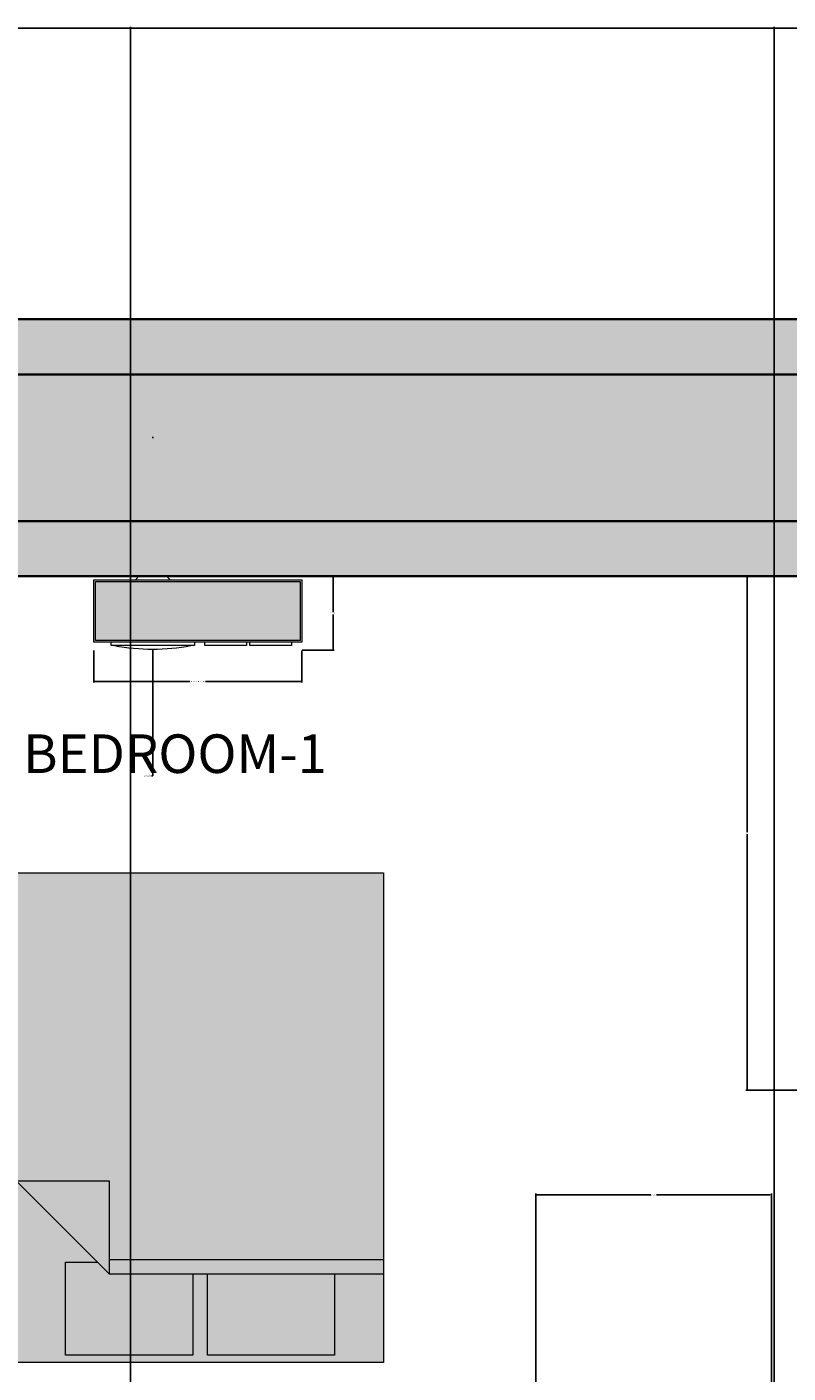
# Model space of a CAD drawing. Units: inches. Extents: x 2549 to 3108, y 1683 to 2362.
# Tile 20 of 30: x 2664 to 2788, y 2142 to 2362. Entities that reach past the tile are written whole.
import ezdxf

# ---------------------------------------------------------------- set-up
doc = ezdxf.new("R2010")
doc.units = ezdxf.units.IN
for name, color, linetype, lineweight in [('A-ANNO-DIMS', 2, 'Continuous', 18), ('A-AREA-IDEN', 7, 'Continuous', 18), ('A-FURN', 8, 'Continuous', 18), ('A-FURN-PATT', 9, 'Continuous', 13), ('A-WALL', 7, 'Continuous', 35), ('A-WALL-PATT', 89, 'Continuous', 13), ('C-PROP', 7, 'Continuous', 35)]:
    doc.layers.add(name, color=color, linetype=linetype, lineweight=lineweight)
for name, color, linetype, lineweight, true_color in [('C-PKNG-VEHI-PATT', 251, 'Continuous', 13, 0x636466), ('C-PROP-PATT', 252, 'Continuous', 13, 0x939598), ('C-PVMT-PATT', 9, 'Continuous', 13, 0xc7c8ca)]:
    doc.layers.add(name, color=color, linetype=linetype, lineweight=lineweight, true_color=true_color)
doc.styles.get("Standard").update_dxf_attribs({"font": 'arial.ttf'})
doc.dimstyles.get("Standard").update_dxf_attribs({"dimtxt": 0.18, "dimasz": 0.18, "dimexe": 0.18, "dimexo": 0.0625, "dimgap": 0.09, "dimtad": 0, "dimtih": 1, "dimtoh": 1, "dimdec": 4, "dimzin": 0, "dimdsep": 46, "dimtxsty": 'Standard', "dimcen": 0.09, "dimadec": 0, "dimazin": 0, "dimtfac": 1, "dimtdec": 4, "dimtofl": 0, "dimtmove": 0, "dimatfit": 3, "dimfxl": 1, "dimtolj": 1, "dimtzin": 0, "dimarcsym": 0})

# ---------------------------------------------------------------- blocks, each defined once
blk = doc.blocks.new('Bed - Queen')
for p, q in [((0, -80.00003), (0, 0)), ((0, 0), (59.99999, 0)), ((59.99999, 0), (59.99999, -80.00003)), ((7.99999, -1.2), (28.79998, -1.2)), ((7.99999, -14.4), (7.99999, -1.2)), ((28.79998, -1.2), (28.79998, -14.4)), ((31.19999, -1.2), (51.99999, -1.2)), ((31.19999, -14.4), (31.19999, -1.2)), ((51.99999, -1.2), (51.99999, -16.4)), ((0, -14.4), (44.8, -14.4)), ((59.99999, -29.6), (44.8, -14.4)), ((44.8, -14.4), (44.8, -29.6)), ((44.8, -16.8), (0, -16.8)), ((51.99999, -16.4), (46.79936, -16.4)), ((44.8, -29.6), (59.99999, -29.6)), ((59.99999, -80.00003), (0, -80.00003))]:
    blk.add_line(p, q)
blk = doc.blocks.new('Entertainment Center')
for p, q in [((-4, 0), (-5, -1)), ((4, 0), (-4, 0)), ((5, -1), (4, 0)), ((-17, -19), (-17, -1)), ((-17, -1), (43, -1)), ((-16.5, -18.5), (-16.5, -1.5)), ((-16.5, -1.5), (42.5, -1.5)), ((42.5, -1.5), (42.5, -18.5)), ((43, -1), (43, -19)), ((43, -19), (-17, -19)), ((42.5, -18.5), (-16.5, -18.5)), ((-12, -20), (-12, -19)), ((12, -19), (12, -20)), ((15, -20), (15, -19)), ((27, -19), (27, -20)), ((28, -20), (28, -19)), ((40, -19), (40, -20)), ((12, -20), (-12, -20)), ((27, -20), (15, -20)), ((40, -20), (28, -20))]:
    blk.add_line(p, q)
blk.add_arc((0, 40), 61, 259.6111, 280.3889)
blk = doc.blocks.new('*D14')
at = {"layer": 'A-ANNO-DIMS', "color": 0, "lineweight": -2, "transparency": 16777216}
for p, q in [((2675, 2260.37), (2675, 2255.15)), ((2709, 2260.37), (2709, 2255.15)), ((2675.18, 2255.33), (2690.71, 2255.33)), ((2708.82, 2255.33), (2693.28, 2255.33))]:
    blk.add_line(p, q, dxfattribs=at)
at = {"layer": 'A-ANNO-DIMS', "color": 0, "transparency": 16777216}
for points in [[(2675.18, 2255.36), (2675.18, 2255.3), (2675, 2255.33)], [(2708.82, 2255.36), (2708.82, 2255.3), (2709, 2255.33)]]:
    blk.add_solid(points, dxfattribs=at)
at = {"layer": 'Defpoints', "color": 0, "transparency": 16777216}
for p in [(2675, 2260.43), (2709, 2260.43), (2709, 2255.33)]:
    blk.add_point(p, dxfattribs=at)
at = {"layer": 'A-ANNO-DIMS', "color": 0, "transparency": 16777216, "insert": (2692, 2255.33), "char_height": 0.18, "attachment_point": 5}
blk.add_mtext('\\A1;MEDIA UNIT 34 TYP.', dxfattribs=at)
blk = doc.blocks.new('*D15')
at = {"layer": 'A-ANNO-DIMS', "color": 0, "lineweight": -2, "transparency": 16777216}
for p, q in [((2709.06, 2272.52), (2714.28, 2272.52)), ((2714.1, 2272.34), (2714.1, 2266.66)), ((2714.1, 2260.61), (2714.1, 2266.3)), ((2709.06, 2260.43), (2714.28, 2260.43))]:
    blk.add_line(p, q, dxfattribs=at)
at = {"layer": 'A-ANNO-DIMS', "color": 0, "transparency": 16777216}
for points in [[(2714.07, 2272.34), (2714.13, 2272.34), (2714.1, 2272.52)], [(2714.07, 2260.61), (2714.13, 2260.61), (2714.1, 2260.43)]]:
    blk.add_solid(points, dxfattribs=at)
at = {"layer": 'Defpoints', "color": 0, "transparency": 16777216}
for p in [(2709, 2272.52), (2714.1, 2272.52), (2709, 2260.43)]:
    blk.add_point(p, dxfattribs=at)
at = {"layer": 'A-ANNO-DIMS', "color": 0, "transparency": 16777216, "insert": (2714.1, 2266.48), "char_height": 0.18, "attachment_point": 5}
blk.add_mtext('\\A1;12 TYP.', dxfattribs=at)
blk = doc.blocks.new('*D27')
at = {"layer": 'A-ANNO-DIMS', "color": 0, "lineweight": -2, "transparency": 16777216}
for p, q in [((2629.64, 2281.59), (2629.64, 2362.32)), ((2629.82, 2362.14), (2720.86, 2362.14)), ((2812.46, 2362.14), (2721.42, 2362.14)), ((2812.64, 2272.59), (2812.64, 2362.32))]:
    blk.add_line(p, q, dxfattribs=at)
at = {"layer": 'A-ANNO-DIMS', "color": 0, "transparency": 16777216}
for points in [[(2629.82, 2362.17), (2629.82, 2362.11), (2629.64, 2362.14)], [(2812.46, 2362.17), (2812.46, 2362.11), (2812.64, 2362.14)]]:
    blk.add_solid(points, dxfattribs=at)
at = {"layer": 'Defpoints', "color": 0, "transparency": 16777216}
for p in [(2812.64, 2362.14), (2629.64, 2281.52), (2812.64, 2272.52)]:
    blk.add_point(p, dxfattribs=at)
at = {"layer": 'A-ANNO-DIMS', "color": 0, "transparency": 16777216, "insert": (2721.14, 2362.14), "char_height": 0.18, "attachment_point": 5}
blk.add_mtext('\\A1;183', dxfattribs=at)
blk = doc.blocks.new('*D37')
at = {"layer": 'A-ANNO-DIMS', "color": 0, "lineweight": -2, "transparency": 16777216}
for p, q in [((2812.58, 2272.52), (2781.56, 2272.52)), ((2781.74, 2272.34), (2781.74, 2230.71)), ((2781.74, 2188.7), (2781.74, 2230.34)), ((2812.58, 2188.52), (2781.56, 2188.52))]:
    blk.add_line(p, q, dxfattribs=at)
at = {"layer": 'A-ANNO-DIMS', "color": 0, "transparency": 16777216}
for points in [[(2781.71, 2272.34), (2781.77, 2272.34), (2781.74, 2272.52)], [(2781.71, 2188.7), (2781.77, 2188.7), (2781.74, 2188.52)]]:
    blk.add_solid(points, dxfattribs=at)
at = {"layer": 'Defpoints', "color": 0, "transparency": 16777216}
for p in [(2781.74, 2272.52), (2812.64, 2272.52), (2812.64, 2188.52)]:
    blk.add_point(p, dxfattribs=at)
at = {"layer": 'A-ANNO-DIMS', "color": 0, "transparency": 16777216, "insert": (2781.74, 2230.52), "char_height": 0.18, "attachment_point": 5}
blk.add_mtext('\\A1;84', dxfattribs=at)
blk = doc.blocks.new('*D40')
at = {"layer": 'A-ANNO-DIMS', "color": 0, "lineweight": -2, "transparency": 16777216}
for p, q in [((2747.21, 2140.59), (2747.21, 2171.6)), ((2747.39, 2171.42), (2766, 2171.42)), ((2785.54, 2171.42), (2766.93, 2171.42)), ((2785.72, 2140.59), (2785.72, 2171.6))]:
    blk.add_line(p, q, dxfattribs=at)
at = {"layer": 'A-ANNO-DIMS', "color": 0, "transparency": 16777216}
for points in [[(2747.39, 2171.45), (2747.39, 2171.39), (2747.21, 2171.42)], [(2785.54, 2171.45), (2785.54, 2171.39), (2785.72, 2171.42)]]:
    blk.add_solid(points, dxfattribs=at)
at = {"layer": 'Defpoints', "color": 0, "transparency": 16777216}
for p in [(2785.72, 2171.42), (2747.21, 2140.52), (2785.72, 2140.52)]:
    blk.add_point(p, dxfattribs=at)
at = {"layer": 'A-ANNO-DIMS', "color": 0, "transparency": 16777216, "insert": (2766.47, 2171.42), "char_height": 0.18, "attachment_point": 5}
blk.add_mtext('\\A1;38.505', dxfattribs=at)
blk = doc.blocks.new('*D59')
at = {"layer": 'A-ANNO-DIMS', "color": 0, "lineweight": -2, "transparency": 16777216}
for p, q in [((2680.98, 1761.59), (2680.98, 2362.32)), ((2681.16, 2362.14), (2733.11, 2362.14)), ((2785.98, 2362.14), (2734.02, 2362.14)), ((2786.16, 1761.59), (2786.16, 2362.32))]:
    blk.add_line(p, q, dxfattribs=at)
at = {"layer": 'A-ANNO-DIMS', "color": 0, "transparency": 16777216}
for points in [[(2681.16, 2362.17), (2681.16, 2362.11), (2680.98, 2362.14)], [(2785.98, 2362.17), (2785.98, 2362.11), (2786.16, 2362.14)]]:
    blk.add_solid(points, dxfattribs=at)
at = {"layer": 'Defpoints', "color": 0, "transparency": 16777216}
for p in [(2786.16, 2362.14), (2680.98, 1761.52), (2786.16, 1761.52)]:
    blk.add_point(p, dxfattribs=at)
at = {"layer": 'A-ANNO-DIMS', "color": 0, "transparency": 16777216, "insert": (2733.57, 2362.14), "char_height": 0.18, "attachment_point": 5}
blk.add_mtext('\\A1;105.18', dxfattribs=at)
blk = doc.blocks.new('*D65')
at = {"layer": 'A-ANNO-DIMS', "color": 0, "lineweight": -2, "transparency": 16777216}
for p, q in [((2684.54, 2295.19), (2684.72, 2295.19)), ((2684.63, 2295.1), (2684.63, 2295.28)), ((2684.63, 2239.88), (2684.63, 2260.44)), ((2684.45, 2239.88), (2684.63, 2239.88))]:
    blk.add_line(p, q, dxfattribs=at)
at = {"layer": 'A-ANNO-DIMS', "color": 0, "transparency": 16777216}
blk.add_solid([(2684.6, 2260.44), (2684.66, 2260.44), (2684.63, 2260.62)], dxfattribs=at)
at = {"layer": 'Defpoints', "color": 0, "transparency": 16777216}
for p in [(2684.63, 2295.19), (2684.63, 2260.62)]:
    blk.add_point(p, dxfattribs=at)
at = {"layer": 'A-ANNO-DIMS', "color": 0, "transparency": 16777216, "insert": (2683.78, 2239.88), "char_height": 0.18, "attachment_point": 5}
blk.add_mtext('\\A1;2X R34.57', dxfattribs=at)

msp = doc.modelspace()

# ---------------------------------------------------------------- hatches: boundary and pattern name
at = {"layer": 'A-FURN-PATT', "transparency": 33554567}
h = msp.add_hatch(color=256, dxfattribs=at)
h.dxf.hatch_style = 1
h.paths.add_polyline_path([(2708.7147, 2271.6737), (2675.2813, 2271.6737), (2675.2813, 2262.0404), (2708.7147, 2262.0404)])
h.paths.add_polyline_path([(2980.8246, 2271.6737), (2947.3913, 2271.6737), (2947.3913, 2262.0404), (2980.8246, 2262.0404)])
h.paths.add_polyline_path([(2748.8496, 2101.6383), (2798.148, 2101.6383), (2798.148, 2111.4248), (2748.8496, 2111.4248)], flags=9)
h.paths.add_polyline_path([(2685.2081, 2101.489), (2719.3253, 2101.489), (2719.3253, 2111.2819), (2685.2081, 2111.2819)], flags=9)
h.paths.add_polyline_path([(2814.6852, 1907.1328), (2847.8384, 1907.1328), (2847.8384, 1916.9258), (2814.6852, 1916.9258)], flags=9)
h.paths.add_polyline_path([(2814.3906, 1835.5864), (2848.0172, 1835.5864), (2848.0172, 1845.3794), (2814.3906, 1845.3794)], flags=9)
h.paths.add_polyline_path([(2800.5245, 1759.1674), (2853.7435, 1759.1674), (2853.7435, 1768.954), (2800.5245, 1768.954)], flags=9)
h.paths.add_polyline_path([(2972.4611, 1807.3305), (3015.3943, 1807.3305), (3015.3943, 1817.117), (2972.4611, 1817.117)], flags=9)
h.paths.add_polyline_path([(2902.3327, 1888.6731), (2937.9131, 1888.6731), (2937.9131, 1898.4661), (2902.3327, 1898.4661)], flags=9)
h.paths.add_polyline_path([(2712.1779, 1878.9039), (2754.1257, 1878.9039), (2754.1257, 1888.6904), (2712.1779, 1888.6904)], flags=9)
h.paths.add_polyline_path([(2614.0056, 2012.812), (2650.0251, 2012.812), (2650.0251, 2022.4371), (2614.0056, 2022.4371)], flags=9)
h.paths.add_polyline_path([(2713.3129, 2003.1645), (2747.4237, 2003.1645), (2747.4237, 2012.951), (2713.3129, 2012.951)], flags=9)
h.paths.add_polyline_path([(2950.1379, 2001.6934), (2982.2992, 2001.6934), (2982.2992, 2011.48), (2950.1379, 2011.48)], flags=9)
h.paths.add_polyline_path([(2940.864, 2238.5537), (2997.5066, 2238.5537), (2997.5066, 2248.3466), (2940.864, 2248.3466)], flags=9)
h.paths.add_polyline_path([(2821.5457, 2202.8348), (2855.663, 2202.8348), (2855.663, 2212.6278), (2821.5457, 2212.6278)], flags=9)
h.paths.add_polyline_path([(2661.8026, 2238.6249), (2718.4451, 2238.6249), (2718.4451, 2248.4179), (2661.8026, 2248.4179)], flags=9)
h = msp.add_hatch(color=256, dxfattribs=at)
h.dxf.hatch_style = 1
h.paths.add_polyline_path([(2906.5064, 1905.2148), (2905.2584, 1904.3827), (2907.0611, 1900.7772), (2908.3092, 1901.6092)])
h.paths.add_polyline_path([(2936.522, 1914.8044), (2935.2739, 1915.6364), (2932.6391, 1912.5856), (2933.8871, 1911.7535)])
h.paths.add_polyline_path([(2950.2508, 1905.6518), (2949.0027, 1906.4839), (2947.1999, 1902.8783), (2948.448, 1902.0463)])
h.paths.add_polyline_path([(2958.5713, 1918.1326), (2956.9072, 1919.242), (2952.4696, 1908.98, 1.38742744), (2954.9657, 1907.3159)])
h.paths.add_polyline_path([(2945.2585, 1927.0078), (2943.5944, 1928.1172), (2934.9965, 1920.6287, 1.38742744), (2937.4927, 1918.9646)])
h.paths.add_polyline_path([(2748.8496, 2101.6383), (2798.148, 2101.6383), (2798.148, 2111.4248), (2748.8496, 2111.4248)], flags=9)
h.paths.add_polyline_path([(2685.2081, 2101.489), (2719.3253, 2101.489), (2719.3253, 2111.2819), (2685.2081, 2111.2819)], flags=9)
h.paths.add_polyline_path([(2814.6852, 1907.1328), (2847.8384, 1907.1328), (2847.8384, 1916.9258), (2814.6852, 1916.9258)], flags=9)
h.paths.add_polyline_path([(2814.3906, 1835.5864), (2848.0172, 1835.5864), (2848.0172, 1845.3794), (2814.3906, 1845.3794)], flags=9)
h.paths.add_polyline_path([(2800.5245, 1759.1674), (2853.7435, 1759.1674), (2853.7435, 1768.954), (2800.5245, 1768.954)], flags=9)
h.paths.add_polyline_path([(2972.4611, 1807.3305), (3015.3943, 1807.3305), (3015.3943, 1817.117), (2972.4611, 1817.117)], flags=9)
h.paths.add_polyline_path([(2902.3327, 1888.6731), (2937.9131, 1888.6731), (2937.9131, 1898.4661), (2902.3327, 1898.4661)], flags=9)
h.paths.add_polyline_path([(2712.1779, 1878.9039), (2754.1257, 1878.9039), (2754.1257, 1888.6904), (2712.1779, 1888.6904)], flags=9)
h.paths.add_polyline_path([(2614.0056, 2012.812), (2650.0251, 2012.812), (2650.0251, 2022.4371), (2614.0056, 2022.4371)], flags=9)
h.paths.add_polyline_path([(2713.3129, 2003.1645), (2747.4237, 2003.1645), (2747.4237, 2012.951), (2713.3129, 2012.951)], flags=9)
h.paths.add_polyline_path([(2950.1379, 2001.6934), (2982.2992, 2001.6934), (2982.2992, 2011.48), (2950.1379, 2011.48)], flags=9)
h.paths.add_polyline_path([(2940.864, 2238.5537), (2997.5066, 2238.5537), (2997.5066, 2248.3466), (2940.864, 2248.3466)], flags=9)
h.paths.add_polyline_path([(2821.5457, 2202.8348), (2855.663, 2202.8348), (2855.663, 2212.6278), (2821.5457, 2212.6278)], flags=9)
h.paths.add_polyline_path([(2661.8026, 2238.6249), (2718.4451, 2238.6249), (2718.4451, 2248.4179), (2661.8026, 2248.4179)], flags=9)
at = {"layer": 'A-FURN-PATT', "transparency": 33554684}
h = msp.add_hatch(color=256, dxfattribs=at)
h.dxf.hatch_style = 1
h.paths.add_polyline_path([(2722.3589, 2224.0179), (2662.3589, 2224.0179), (2662.3589, 2173.6179), (2677.5589, 2173.6179), (2677.5589, 2160.8179), (2722.3589, 2160.8179)])
h.paths.add_polyline_path([(2996.4972, 2224.0179), (2936.4972, 2224.0179), (2936.4972, 2173.6179), (2951.6972, 2173.6179), (2951.6972, 2160.8179), (2996.4972, 2160.8179)])
h = msp.add_hatch(color=256, dxfattribs=at)
h.dxf.hatch_style = 1
h.paths.add_polyline_path([(2677.5589, 2173.6179), (2662.3589, 2173.6179), (2677.5589, 2158.4179)], flags=17)
h.paths.add_polyline_path([(2662.3589, 2173.6179), (2662.3589, 2144.0179), (2722.3589, 2144.0179), (2722.3589, 2158.4179), (2714.3589, 2158.4179), (2714.3589, 2145.2179), (2693.5589, 2145.2179), (2693.5589, 2158.4179), (2691.1589, 2158.4179), (2691.1589, 2145.2179), (2670.3589, 2145.2179), (2670.3589, 2160.4179), (2675.5589, 2160.4179)])
h.paths.add_polyline_path([(2722.3589, 2160.8179), (2677.5589, 2160.8179), (2677.5589, 2158.4179), (2722.3589, 2158.4179)], flags=17)
h.paths.add_polyline_path([(2951.6972, 2173.6179), (2936.4972, 2173.6179), (2951.6972, 2158.4179)], flags=17)
h.paths.add_polyline_path([(2936.4972, 2173.6179), (2936.4972, 2144.0179), (2996.4972, 2144.0179), (2996.4972, 2158.4179), (2988.4972, 2158.4179), (2988.4972, 2145.2179), (2967.6972, 2145.2179), (2967.6972, 2158.4179), (2965.2972, 2158.4179), (2965.2972, 2145.2179), (2944.4972, 2145.2179), (2944.4972, 2160.4179), (2949.6972, 2160.4179)])
h.paths.add_polyline_path([(2996.4972, 2160.8179), (2951.6972, 2160.8179), (2951.6972, 2158.4179), (2996.4972, 2158.4179)], flags=17)
h = msp.add_hatch(color=256, dxfattribs=at)
h.dxf.hatch_style = 1
h.paths.add_polyline_path([(2691.1589, 2158.4179), (2677.5589, 2158.4179), (2675.5589, 2160.4179), (2670.3589, 2160.4179), (2670.3589, 2145.2179), (2691.1589, 2145.2179)])
h.paths.add_polyline_path([(2714.3589, 2158.4179), (2693.5589, 2158.4179), (2693.5589, 2145.2179), (2714.3589, 2145.2179)])
h.paths.add_polyline_path([(2965.2972, 2158.4179), (2951.6972, 2158.4179), (2949.6972, 2160.4179), (2944.4972, 2160.4179), (2944.4972, 2145.2179), (2965.2972, 2145.2179)])
h.paths.add_polyline_path([(2988.4972, 2158.4179), (2967.6972, 2158.4179), (2967.6972, 2145.2179), (2988.4972, 2145.2179)])
at = {"layer": 'A-WALL-PATT'}
h = msp.add_hatch(color=256, dxfattribs=at)
h.dxf.hatch_style = 1
h.paths.add_polyline_path([(2638.6427, 2272.5237), (3034.6427, 2272.5237), (3034.6427, 1936.5237), (3043.6427, 1936.5237), (3043.6427, 2281.5237), (2629.6427, 2281.5237), (2629.6427, 2074.5237), (2812.6427, 2074.5237), (2812.6427, 2140.5237), (2785.7177, 2140.5237), (2785.7177, 2134.5237), (2806.6427, 2134.5237), (2806.6427, 2080.5237), (2638.6427, 2080.5237)])
h.paths.add_polyline_path([(2638.6427, 1972.5237), (2662.6427, 1972.5237), (2662.6427, 2041.0557), (2653.6427, 2041.0557), (2653.6427, 1978.5237), (2629.6427, 1978.5237), (2629.6427, 1795.5237), (2662.6427, 1795.5237), (2881.6427, 1795.5237), (2881.6427, 1936.5237), (2965.9351, 1936.5237), (2965.9351, 1974.5439), (2959.9351, 1974.5439), (2959.9351, 1945.5237), (2881.6427, 1945.5237), (2872.6427, 1945.5237), (2872.6427, 1804.5237), (2662.6427, 1804.5237), (2638.6427, 1804.5237)])
at = {"layer": 'C-PKNG-VEHI-PATT'}
h = msp.add_hatch(color=256, dxfattribs=at)
h.dxf.hatch_style = 1
edge = h.paths.add_edge_path()
edge.add_ellipse((2935.7258, 1791.964), major_axis=(-50.66, 0), ratio=0.84230387, start_angle=248.165046, end_angle=265.722579)
edge.add_line((2938.911, 1834.5507), (2925.8653, 1834.5507))
edge.add_ellipse((2929.0505, 1791.964), major_axis=(50.66, 0), ratio=0.84230387, start_angle=94.277421, end_angle=111.834954)
edge.add_line((2912.8508, 1832.3947), (2914.2044, 1822.2495))
edge.add_ellipse((2930.6538, 1783.1023), major_axis=(-49.3014, 0), ratio=0.84230387, start_angle=-85.12993, end_angle=-67.208085, ccw=False)
edge.add_line((2927.1247, 1824.5225), (2937.6516, 1824.5225))
edge.add_ellipse((2934.1225, 1783.1023), major_axis=(49.3014, 0), ratio=0.84230387, start_angle=67.208085, end_angle=85.12993, ccw=False)
edge.add_line((2950.5719, 1822.2495), (2951.9255, 1832.3947))
edge = h.paths.add_edge_path()
edge.add_ellipse((2903.4793, 1857.3351), major_axis=(-34.7979, 0), ratio=0.84230387, start_angle=180, end_angle=209.43857)
edge.add_ellipse((2961.297, 1857.3351), major_axis=(34.7979, 0), ratio=0.84230387, start_angle=150.56143, end_angle=180)
edge.add_line((2926.4991, 1857.3351), (2926.4991, 1843.7609))
edge.add_ellipse((2924.1251, 1844.3143), major_axis=(-0.2209, 3.9278), ratio=0.60383358, start_angle=89.002014, end_angle=253.657408, ccw=False)
edge.add_line((2921.7512, 1844.2222), (2921.7512, 1853.3975))
edge.add_line((2921.7512, 1853.3975), (2925.269, 1855.8484))
edge.add_ellipse((2925.4782, 1855.4931), major_axis=(0.4584, 0), ratio=0.84230387, start_angle=90, end_angle=134.480211, ccw=False)
edge.add_line((2925.4782, 1855.8792), (2926.4991, 1855.8792))
edge.add_line((2926.4991, 1855.8792), (2926.4991, 1857.3351))
edge.add_ellipse((2961.297, 1857.3351), major_axis=(34.7979, 0), ratio=0.84230387, start_angle=150.56143, end_angle=180, ccw=False)
edge.add_line((2932.3882, 1873.6501), (2932.3882, 1875.7801))
edge.add_ellipse((2932.3882, 1875.3939), major_axis=(0.4584, 0), ratio=0.84230387, start_angle=90, end_angle=127.93313)
edge.add_line((2932.1366, 1875.7167), (2928.5915, 1873.7564))
edge.add_ellipse((2899.9271, 2002.4692), major_axis=(155.4756, 0), ratio=0.84230387, start_angle=-80.743434, end_angle=-77.445067, ccw=False)
edge.add_ellipse((2949.4402, 1715.2151), major_axis=(-189.1422, 0), ratio=0.84230387, start_angle=-79.790461, end_angle=-77.555373)
edge.add_ellipse((3300.3614, 1852.5642), major_axis=(-386.1662, 0), ratio=0.84230387, start_angle=-2.863715, end_angle=2.198541)
edge.add_ellipse((2929.0505, 1792.5159), major_axis=(-55.6192, 0), ratio=0.84230387, start_angle=-85.917589, end_angle=-72.280047, ccw=False)
edge.add_line((2925.7129, 1839.2798), (2939.0634, 1839.2798))
edge.add_ellipse((2935.7258, 1792.5159), major_axis=(55.6192, 0), ratio=0.84230387, start_angle=72.280047, end_angle=85.917589, ccw=False)
edge.add_ellipse((2564.4149, 1852.5642), major_axis=(-386.1662, 0), ratio=0.84230387, start_angle=177.801459, end_angle=182.863715)
edge.add_ellipse((2915.3361, 1715.2151), major_axis=(189.1422, 0), ratio=0.84230387, start_angle=77.555373, end_angle=79.790461)
edge.add_ellipse((2964.8492, 2002.4692), major_axis=(-155.4756, 0), ratio=0.84230387, start_angle=77.445067, end_angle=80.743434, ccw=False)
edge.add_line((2936.1848, 1873.7564), (2932.6397, 1875.7167))
edge.add_ellipse((2932.3882, 1875.3939), major_axis=(0.4584, 0), ratio=0.84230387, start_angle=52.06687, end_angle=90)
edge.add_line((2932.3882, 1875.7801), (2932.3882, 1873.6501))
edge.add_ellipse((2903.4793, 1857.3351), major_axis=(-34.7979, 0), ratio=0.84230387, start_angle=180, end_angle=209.43857, ccw=False)
edge.add_line((2938.2772, 1857.3351), (2938.2772, 1855.8792))
edge.add_line((2938.2772, 1855.8792), (2939.4059, 1855.8792))
edge.add_ellipse((2939.2981, 1855.4931), major_axis=(-0.4584, 0), ratio=0.84230387, start_angle=225.519789, end_angle=270, ccw=False)
edge.add_line((2939.5903, 1855.7906), (2943.0251, 1853.3975))
edge.add_line((2943.0251, 1853.3975), (2943.0251, 1844.2222))
edge.add_ellipse((2940.6512, 1844.3143), major_axis=(0.2209, 3.9278), ratio=0.60383358, start_angle=106.342592, end_angle=270.997986, ccw=False)
edge.add_line((2938.2772, 1843.7609), (2938.2772, 1857.3351))
edge = h.paths.add_edge_path()
edge.add_ellipse((2932.3882, 1865.1973), major_axis=(91.081, 0), ratio=0.84230387, start_angle=256.401865, end_angle=283.598135, ccw=False)
edge.add_line((2914.2044, 1790.0239), (2914.2044, 1778.3622))
edge.add_ellipse((2932.3882, 1853.5356), major_axis=(91.081, 0), ratio=0.84230387, start_angle=256.401865, end_angle=283.598135)
edge.add_line((2950.5719, 1778.3622), (2950.5719, 1790.0239))
edge = h.paths.add_edge_path()
edge.add_ellipse((2948.7383, 1772.3145), major_axis=(1.8336, 0), ratio=0.84230387, start_angle=0, end_angle=90)
edge.add_line((2948.7383, 1773.859), (2916.038, 1773.859))
edge.add_ellipse((2916.038, 1772.3145), major_axis=(1.8336, 0), ratio=0.84230387, start_angle=90, end_angle=180)
edge.add_line((2914.2044, 1772.3145), (2914.2044, 1760.2558))
edge.add_line((2914.2044, 1760.2558), (2950.5719, 1760.2558))
edge.add_line((2950.5719, 1760.2558), (2950.5719, 1772.3145))
h.paths.add_polyline_path([(2748.8496, 2101.6383), (2798.148, 2101.6383), (2798.148, 2111.4248), (2748.8496, 2111.4248)], flags=9)
h.paths.add_polyline_path([(2685.2081, 2101.489), (2719.3253, 2101.489), (2719.3253, 2111.2819), (2685.2081, 2111.2819)], flags=9)
h.paths.add_polyline_path([(2814.6852, 1907.1328), (2847.8384, 1907.1328), (2847.8384, 1916.9258), (2814.6852, 1916.9258)], flags=9)
h.paths.add_polyline_path([(2814.3906, 1835.5864), (2848.0172, 1835.5864), (2848.0172, 1845.3794), (2814.3906, 1845.3794)], flags=9)
h.paths.add_polyline_path([(2800.5245, 1759.1674), (2853.7435, 1759.1674), (2853.7435, 1768.954), (2800.5245, 1768.954)], flags=9)
h.paths.add_polyline_path([(2972.4611, 1807.3305), (3015.3943, 1807.3305), (3015.3943, 1817.117), (2972.4611, 1817.117)], flags=9)
h.paths.add_polyline_path([(2902.3327, 1888.6731), (2937.9131, 1888.6731), (2937.9131, 1898.4661), (2902.3327, 1898.4661)], flags=9)
h.paths.add_polyline_path([(2712.1779, 1878.9039), (2754.1257, 1878.9039), (2754.1257, 1888.6904), (2712.1779, 1888.6904)], flags=9)
h.paths.add_polyline_path([(2614.0056, 2012.812), (2650.0251, 2012.812), (2650.0251, 2022.4371), (2614.0056, 2022.4371)], flags=9)
h.paths.add_polyline_path([(2713.3129, 2003.1645), (2747.4237, 2003.1645), (2747.4237, 2012.951), (2713.3129, 2012.951)], flags=9)
h.paths.add_polyline_path([(2950.1379, 2001.6934), (2982.2992, 2001.6934), (2982.2992, 2011.48), (2950.1379, 2011.48)], flags=9)
h.paths.add_polyline_path([(2940.864, 2238.5537), (2997.5066, 2238.5537), (2997.5066, 2248.3466), (2940.864, 2248.3466)], flags=9)
h.paths.add_polyline_path([(2821.5457, 2202.8348), (2855.663, 2202.8348), (2855.663, 2212.6278), (2821.5457, 2212.6278)], flags=9)
h.paths.add_polyline_path([(2661.8026, 2238.6249), (2718.4451, 2238.6249), (2718.4451, 2248.4179), (2661.8026, 2248.4179)], flags=9)
at = {"layer": 'C-PROP-PATT'}
h = msp.add_hatch(color=256, dxfattribs=at)
h.dxf.hatch_style = 1
h.paths.add_polyline_path([(3076.6427, 2314.5237), (2596.6427, 2314.5237), (2596.6427, 1714.5237), (2881.84, 1714.5237), (2881.84, 1723.5237), (2605.6427, 1723.5237), (2605.6427, 2305.5237), (3067.6427, 2305.5237), (3067.6427, 1723.5237), (3067.6427, 1714.5237), (3076.6427, 1714.5237)])
at = {"layer": 'C-PVMT-PATT'}
h = msp.add_hatch(color=256, dxfattribs=at)
h.dxf.hatch_style = 1
h.paths.add_polyline_path([(3067.6427, 2305.5237), (2605.6427, 2305.5237), (2605.6427, 2074.5237), (2629.6427, 2074.5237), (2629.6427, 2281.5237), (3043.6427, 2281.5237), (3043.6427, 1885.5237), (3043.6427, 1872.8745), (3031.1672, 1872.8745), (3031.1672, 1862.5731), (2995.8054, 1862.5731), (2995.8054, 1872.8745), (2983.1752, 1872.8745), (2983.1752, 1885.5237), (2881.6427, 1885.5237), (2881.6427, 1795.5237), (2751.0977, 1795.5237), (2751.0977, 1761.5237), (2786.1577, 1761.5237), (2786.1577, 1723.5237), (2881.84, 1723.5237), (2881.84, 1714.5237), (3067.6427, 1714.5237), (3067.6427, 1723.5237)])
edge = h.paths.add_edge_path(flags=16)
edge.add_ellipse((2949.4402, 1710.9683), major_axis=(-194.1014, 0), ratio=0.84230387, start_angle=-77.874034, end_angle=-76.219471, ccw=False)
edge.add_ellipse((2949.4402, 1715.2151), major_axis=(-189.1422, 0), ratio=0.84230387, start_angle=-79.790461, end_angle=-77.555373, ccw=False)
edge.add_ellipse((2899.9271, 2002.4692), major_axis=(155.4756, 0), ratio=0.84230387, start_angle=-80.743434, end_angle=-77.445067)
edge.add_line((2928.5915, 1873.7564), (2932.3882, 1875.8558))
edge.add_line((2932.3882, 1875.8558), (2936.1848, 1873.7564))
edge.add_ellipse((2964.8492, 2002.4692), major_axis=(-155.4756, 0), ratio=0.84230387, start_angle=77.445067, end_angle=80.743434)
edge.add_ellipse((2915.3361, 1715.2151), major_axis=(189.1422, 0), ratio=0.84230387, start_angle=77.555373, end_angle=79.790461, ccw=False)
edge.add_ellipse((2915.3361, 1710.9683), major_axis=(-194.1014, 0), ratio=0.84230387, start_angle=256.219471, end_angle=257.874034, ccw=False)
edge.add_ellipse((2628.2871, 1850.2612), major_axis=(-327.2532, 0), ratio=0.84230387, start_angle=182.17995, end_angle=183.650428, ccw=False)
edge.add_ellipse((2955.5637, 1861.9334), major_axis=(-0.9168, 0), ratio=0.84230387, start_angle=180, end_angle=270, ccw=False)
edge.add_line((2956.4805, 1862.3857), (2956.4805, 1846.4866))
edge.add_ellipse((2955.5637, 1846.939), major_axis=(-0.9168, 0), ratio=0.84230387, start_angle=90, end_angle=180, ccw=False)
edge.add_ellipse((-3607.0606, 1835.832), major_axis=(-6562.6242, 0), ratio=0.84230387, start_angle=179.61613322, end_angle=180.09022909, ccw=False)
edge.add_ellipse((2955.5637, 1791.0926), major_axis=(0.9168, 0), ratio=0.84230387, start_angle=0, end_angle=90, ccw=False)
edge.add_line((2956.4805, 1791.545), (2956.4805, 1775.6459))
edge.add_ellipse((2955.5637, 1776.0982), major_axis=(0.9168, 0), ratio=0.84230387, start_angle=270, end_angle=360, ccw=False)
edge.add_ellipse((-3607.0606, 1835.832), major_axis=(-6562.6242, 0), ratio=0.84230387, start_angle=179.3813568, end_angle=179.47172853, ccw=False)
edge.add_ellipse((2954.5907, 1763.8768), major_axis=(-1.3752, 0), ratio=0.84230387, start_angle=179.371763, end_angle=248.464757, ccw=False)
edge.add_ellipse((-3607.519, 1835.832), major_axis=(-6564.0409, 0), ratio=0.842303863, start_angle=179.35344594, end_angle=179.37176282, ccw=False)
edge.add_ellipse((2952.6829, 1761.8002), major_axis=(3.2503, 0), ratio=0.84230387, start_angle=-90, end_angle=-0.646554, ccw=False)
edge.add_line((2952.6829, 1759.0625), (2912.0934, 1759.0625))
edge.add_ellipse((2912.0934, 1761.8002), major_axis=(3.2503, 0), ratio=0.84230387, start_angle=180.646554, end_angle=270, ccw=False)
edge.add_ellipse((9472.2953, 1835.832), major_axis=(-6564.0409, 0), ratio=0.842303871, start_angle=0.62823722, end_angle=0.6465541, ccw=False)
edge.add_ellipse((2910.1856, 1763.8768), major_axis=(1.3752, 0), ratio=0.84230387, start_angle=111.535244, end_angle=180.628237, ccw=False)
edge.add_ellipse((9471.8369, 1835.832), major_axis=(-6562.6242, 0), ratio=0.84230387, start_angle=0.52827147, end_angle=0.6465541, ccw=False)
edge.add_ellipse((2909.2126, 1776.0982), major_axis=(-0.9168, 0), ratio=0.84230387, start_angle=0, end_angle=90, ccw=False)
edge.add_line((2908.2958, 1775.6459), (2908.2958, 1791.545))
edge.add_ellipse((2909.2126, 1791.0926), major_axis=(-0.9168, 0), ratio=0.84230387, start_angle=-90, end_angle=0, ccw=False)
edge.add_ellipse((9471.8369, 1835.832), major_axis=(-6562.6242, 0), ratio=0.84230387, start_angle=-0.09022909, end_angle=0.38386678, ccw=False)
edge.add_ellipse((2909.2126, 1846.939), major_axis=(-0.9168, 0), ratio=0.84230387, start_angle=0, end_angle=90, ccw=False)
edge.add_line((2908.2958, 1846.4866), (2908.2958, 1862.3857))
edge.add_ellipse((2909.2126, 1861.9334), major_axis=(0.9168, 0), ratio=0.84230387, start_angle=90, end_angle=180, ccw=False)
edge.add_ellipse((3236.4892, 1850.2612), major_axis=(327.2532, 0), ratio=0.84230387, start_angle=176.349572, end_angle=177.82005, ccw=False)
edge = h.paths.add_edge_path(flags=0)
edge.add_ellipse((2903.4793, 1857.3351), major_axis=(-34.7979, 0), ratio=0.84230387, start_angle=180, end_angle=209.43857, ccw=False)
edge.add_line((2938.2772, 1857.3351), (2938.2772, 1855.8792))
edge.add_line((2938.2772, 1855.8792), (2939.4631, 1855.8792))
edge.add_line((2939.4631, 1855.8792), (2943.0251, 1853.3975))
edge.add_line((2943.0251, 1853.3975), (2943.0251, 1844.2222))
edge.add_ellipse((2940.6512, 1844.3143), major_axis=(0.2209, 3.9278), ratio=0.60383358, start_angle=106.342592, end_angle=270.997986, ccw=False)
edge.add_line((2938.2772, 1843.7609), (2938.2772, 1857.3351))
edge.add_ellipse((2903.4793, 1857.3351), major_axis=(-34.7979, 0), ratio=0.84230387, start_angle=180, end_angle=209.43857)
edge.add_ellipse((2961.297, 1857.3351), major_axis=(34.7979, 0), ratio=0.84230387, start_angle=150.56143, end_angle=180)
edge.add_line((2926.4991, 1857.3351), (2926.4991, 1843.7609))
edge.add_ellipse((2924.1251, 1844.3143), major_axis=(-0.2209, 3.9278), ratio=0.60383358, start_angle=89.002014, end_angle=253.657408, ccw=False)
edge.add_line((2921.7512, 1844.2222), (2921.7512, 1853.3975))
edge.add_line((2921.7512, 1853.3975), (2925.3132, 1855.8792))
edge.add_line((2925.3132, 1855.8792), (2926.4991, 1855.8792))
edge.add_line((2926.4991, 1855.8792), (2926.4991, 1857.3351))
edge.add_ellipse((2961.297, 1857.3351), major_axis=(34.7979, 0), ratio=0.84230387, start_angle=150.56143, end_angle=180, ccw=False)
edge = h.paths.add_edge_path(flags=0)
edge.add_ellipse((2929.0505, 1791.964), major_axis=(50.66, 0), ratio=0.84230387, start_angle=94.277421, end_angle=111.834954, ccw=False)
edge.add_line((2925.8653, 1834.5507), (2938.911, 1834.5507))
edge.add_ellipse((2935.7258, 1791.964), major_axis=(-50.66, 0), ratio=0.84230387, start_angle=248.165046, end_angle=265.722579, ccw=False)
edge.add_line((2951.9255, 1832.3947), (2950.5719, 1822.2495))
edge.add_ellipse((2934.1225, 1783.1023), major_axis=(49.3014, 0), ratio=0.84230387, start_angle=67.208085, end_angle=85.12993)
edge.add_line((2937.6516, 1824.5225), (2927.1247, 1824.5225))
edge.add_ellipse((2930.6538, 1783.1023), major_axis=(-49.3014, 0), ratio=0.84230387, start_angle=-85.12993, end_angle=-67.208085)
edge.add_line((2914.2044, 1822.2495), (2912.8508, 1832.3947))
edge = h.paths.add_edge_path(flags=0)
edge.add_line((2910.1338, 1829.4651), (2912.6432, 1821.2711))
edge.add_ellipse((5203.7787, 1816.4367), major_axis=(-2291.1426, 0), ratio=0.84230387, start_angle=-0.1208974, end_angle=0.3640763)
edge.add_line((2912.7012, 1801.8782), (2910.3305, 1792.5698))
edge.add_ellipse((9471.8369, 1835.832), major_axis=(-6561.7074, 0), ratio=0.84230387, start_angle=0.05559431, end_angle=0.37776419, ccw=False)
edge = h.paths.add_edge_path(flags=0)
edge.add_ellipse((-3607.0606, 1835.832), major_axis=(6561.7074, 0), ratio=0.84230387, start_angle=-0.37776419, end_angle=-0.05559431, ccw=False)
edge.add_line((2954.4458, 1792.5698), (2952.0751, 1801.8782))
edge.add_ellipse((660.9976, 1816.4367), major_axis=(2291.1426, 0), ratio=0.84230387, start_angle=-0.3640763, end_angle=0.1208974)
edge.add_line((2952.1331, 1821.2711), (2954.6425, 1829.4651))
edge = h.paths.add_edge_path(flags=0)
edge.add_ellipse((2932.3882, 1865.1973), major_axis=(91.081, 0), ratio=0.84230387, start_angle=256.401865, end_angle=283.598135)
edge.add_line((2950.5719, 1790.0239), (2950.5719, 1778.3622))
edge.add_ellipse((2932.3882, 1853.5356), major_axis=(91.081, 0), ratio=0.84230387, start_angle=256.401865, end_angle=283.598135, ccw=False)
edge.add_line((2914.2044, 1778.3622), (2914.2044, 1790.0239))
edge = h.paths.add_edge_path(flags=0)
edge.add_line((2916.038, 1773.859), (2948.7383, 1773.859))
edge.add_ellipse((2948.7383, 1772.3145), major_axis=(1.8336, 0), ratio=0.84230387, start_angle=0, end_angle=90, ccw=False)
edge.add_line((2950.5719, 1772.3145), (2950.5719, 1760.2558))
edge.add_line((2950.5719, 1760.2558), (2914.2044, 1760.2558))
edge.add_line((2914.2044, 1760.2558), (2914.2044, 1772.3145))
edge.add_ellipse((2916.038, 1772.3145), major_axis=(1.8336, 0), ratio=0.84230387, start_angle=90, end_angle=180, ccw=False)
h.paths.add_polyline_path([(2629.6427, 1978.5237), (2605.6427, 1978.5237), (2605.6427, 1723.5237), (2629.6427, 1723.5237), (2629.6427, 1795.5237)], flags=17)
h.paths.add_polyline_path([(2800.5245, 1759.1674), (2853.7435, 1759.1674), (2853.7435, 1768.954), (2800.5245, 1768.954)], flags=24)
h.paths.add_polyline_path([(2972.4611, 1807.3305), (3015.3943, 1807.3305), (3015.3943, 1817.117), (2972.4611, 1817.117)], flags=24)

# ---------------------------------------------------------------- linework, layer by layer
at = {"layer": 'A-WALL'}
for p, q in [((2629.6427, 2281.5237), (3043.6427, 2281.5237)), ((2638.6427, 2272.5237), (3034.6427, 2272.5237))]:
    msp.add_line(p, q, dxfattribs=at)
at = {"layer": 'C-PROP'}
msp.add_lwpolyline([(2596.6427, 2314.5237), (3076.6427, 2314.5237), (3076.6427, 1714.5237), (2596.6427, 1714.5237)], close=True, dxfattribs=at)
msp.add_lwpolyline([(2881.84, 1723.5237), (2605.6427, 1723.5237), (2605.6427, 2305.5237), (3067.6427, 2305.5237), (3067.6427, 1723.5237)], dxfattribs=at)

# ---------------------------------------------------------------- block references
at = {"layer": 'A-FURN', "xscale": 0.5666666666666667, "yscale": 0.5666666666666667, "zscale": 0.5666666666666667}
msp.add_blockref('Entertainment Center', (2684.6313, 2272.5237), dxfattribs=at)
at = {"layer": 'A-FURN', "rotation": 180}
msp.add_blockref('Bed - Queen', (2722.3589, 2144.0179), dxfattribs=at)

# ---------------------------------------------------------------- texts
at = {"layer": 'A-AREA-IDEN'}
msp.add_text('BEDROOM-1', height=6.30916, dxfattribs=at).set_placement((2663.4347, 2240.3647))

# ---------------------------------------------------------------- dimensions: what is measured, and where the dimension line sits
at = {"layer": 'A-ANNO-DIMS'}
for base, p1, p2, override, picture, middle in [((2812.6427, 2362.1425), (2629.6427, 2281.5237), (2812.6427, 2272.5237), {"dimdec": 0, "dimlfac": 1, "dimrnd": 0, "dimzin": 0, "dimdsep": 46, "dimlunit": 2}, '*D27', (2721.1427, 2362.1425)), ((2786.1577, 2362.1425), (2680.9778, 1761.5237), (2786.1577, 1761.5237), {"dimdec": 2, "dimlfac": 1, "dimrnd": 0, "dimzin": 0, "dimdsep": 46, "dimlunit": 2}, '*D59', (2733.5678, 2362.1425)), ((2785.7177, 2171.4237), (2747.213, 2140.5237), (2785.7177, 2140.5237), {"dimdec": 3, "dimlfac": 1, "dimrnd": 0, "dimzin": 0, "dimdsep": 46, "dimlunit": 2}, '*D40', (2766.4653, 2171.4237))]:
    dim = msp.add_linear_dim(base=base, p1=p1, p2=p2, dimstyle='Standard', override=override, dxfattribs=at)
    dim.commit()
    dim.dimension.update_dxf_attribs({"geometry": picture, "text_midpoint": middle})
dim = msp.add_radius_dim(center=(2684.6313, 2295.1904), mpoint=(2684.631, 2260.6237), text='2X <>', dimstyle='Standard', override={"dimdec": 2, "dimlfac": 1, "dimrnd": 0, "dimzin": 0, "dimdsep": 46, "dimlunit": 2}, dxfattribs=at)
dim.commit()
dim.dimension.update_dxf_attribs({"geometry": '*D65', "text_midpoint": (2683.776, 2239.8837), "dimtype": 164})
dim = msp.add_linear_dim(base=(2714.098, 2272.5237), p1=(2708.998, 2260.4349), p2=(2708.998, 2272.5237), angle=90, text='<> TYP.', dimstyle='Standard', override={"dimdec": 0, "dimlfac": 1, "dimrnd": 0, "dimzin": 0, "dimdsep": 46, "dimlunit": 2}, dxfattribs=at)
dim.commit()
dim.dimension.update_dxf_attribs({"geometry": '*D15', "text_midpoint": (2714.098, 2266.4793)})
dim = msp.add_linear_dim(base=(2781.7427, 2272.5237), p1=(2812.6427, 2188.5237), p2=(2812.6427, 2272.5237), angle=90, dimstyle='Standard', override={"dimdec": 0, "dimlfac": 1, "dimrnd": 0, "dimzin": 0, "dimdsep": 46, "dimlunit": 2}, dxfattribs=at)
dim.commit()
dim.dimension.update_dxf_attribs({"geometry": '*D37', "text_midpoint": (2781.7427, 2230.5237)})
dim = msp.add_linear_dim(base=(2708.998, 2255.3349), p1=(2674.998, 2260.4349), p2=(2708.998, 2260.4349), text='MEDIA UNIT <> TYP.', dimstyle='Standard', override={"dimdec": 0, "dimlfac": 1, "dimrnd": 0, "dimzin": 0, "dimdsep": 46, "dimlunit": 2}, dxfattribs=at)
dim.commit()
dim.dimension.update_dxf_attribs({"geometry": '*D14', "text_midpoint": (2691.998, 2255.3349)})

doc.saveas('drawing.dxf')
